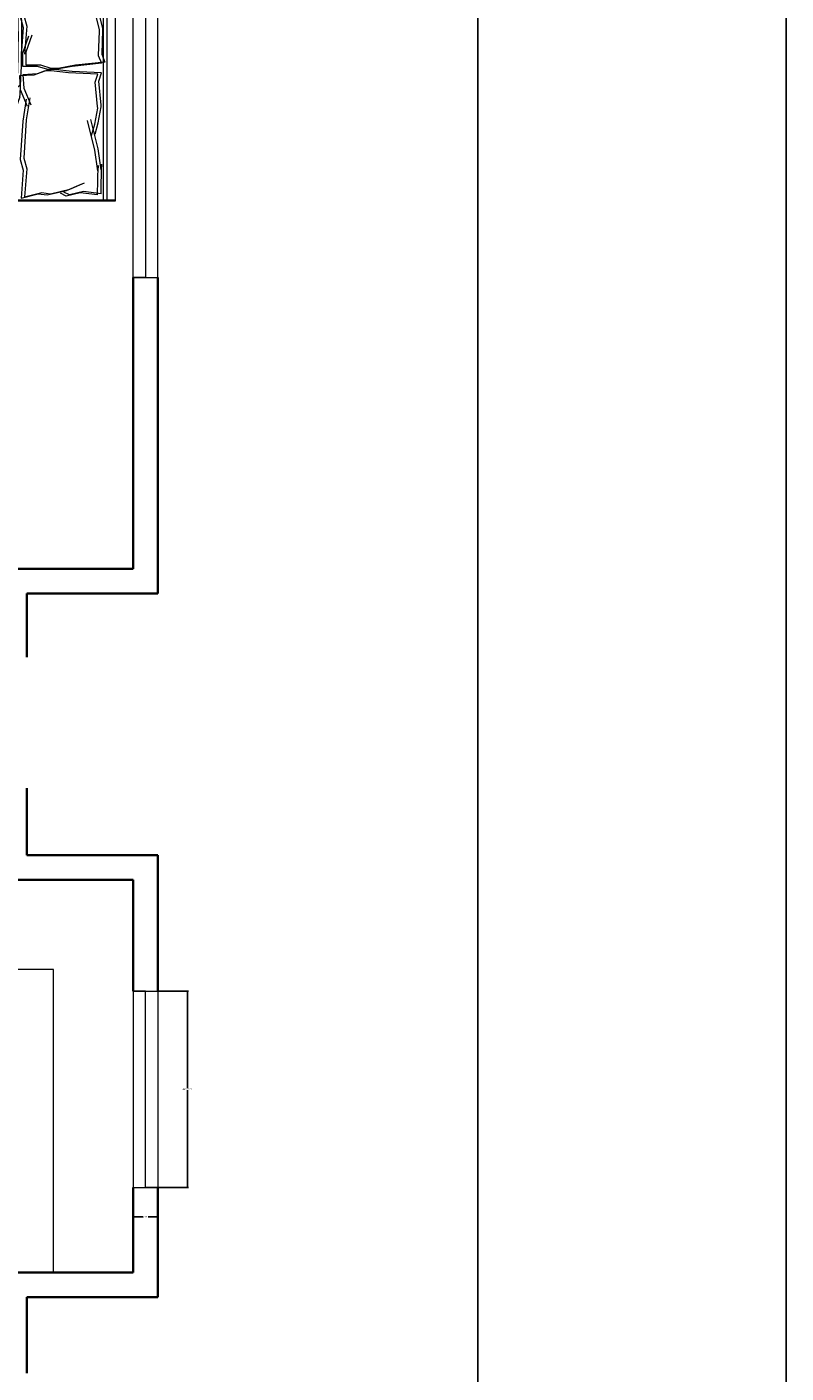
# Model space of a CAD drawing. Units: inches. Extents: x 2163 to 2982, y 1024 to 2288.
# Tile 8 of 22: x 2843 to 2982, y 1390 to 1637. Entities that reach past the tile are written whole.
import ezdxf

# ---------------------------------------------------------------- set-up
doc = ezdxf.new("R2010")
doc.units = ezdxf.units.IN
for name, color, linetype, lineweight in [('A-ANNO-DIMS', 2, 'Continuous', 18), ('A-ANNO-TTLB', 7, 'Continuous', 25), ('A-FLOR-FIXT', 9, 'Continuous', 18), ('A-FURN', 8, 'Continuous', 13), ('A-GLAZ', 161, 'Continuous', 18), ('A-WALL', 7, 'Continuous', 35)]:
    doc.layers.add(name, color=color, linetype=linetype, lineweight=lineweight)
doc.styles.get("Standard").update_dxf_attribs({"font": 'arial.ttf'})
doc.dimstyles.get("Standard").update_dxf_attribs({"dimtxt": 0.18, "dimasz": 0.18, "dimexe": 0.18, "dimexo": 0.0625, "dimgap": 0.09, "dimtad": 0, "dimtih": 1, "dimtoh": 1, "dimdec": 4, "dimzin": 0, "dimdsep": 46, "dimtxsty": 'Standard', "dimcen": 0.09, "dimadec": 0, "dimazin": 0, "dimtfac": 1, "dimtdec": 4, "dimtofl": 0, "dimtmove": 0, "dimatfit": 3, "dimfxl": 1, "dimtolj": 1, "dimtzin": 0, "dimarcsym": 0})

# ---------------------------------------------------------------- blocks, each defined once
blk = doc.blocks.new('BED-DOUBLE')
for p, q in [((27.75, 52.87), (24.5, 49.16)), ((27.75, 52.87), (24.5, 49.16)), ((28.38, 53.1), (25.13, 49.39)), ((28.38, 53.1), (25.13, 49.39)), ((29.49, 52.95), (27.75, 52.87, 3.87)), ((29.49, 52.95), (27.75, 52.87, 3.87)), ((28.36, 51.33), (27.75, 52.87)), ((28.36, 51.33), (27.75, 52.87)), ((30.13, 53.18), (28.38, 53.1, 3.87)), ((29, 51.56), (28.38, 53.1)), ((30.13, 53.18), (28.38, 53.1, 3.87)), ((29, 51.56), (28.38, 53.1)), ((0, 51.49), (0.64, 51.49)), ((0, 3.47), (0, 51.49)), ((0, 51.27), (26.61, 51.27)), ((0, 51.27), (26.61, 51.27)), ((0.64, 51.49), (27.25, 51.49)), ((0.64, 51.49), (27.25, 51.49)), ((1.53, 3.48), (1.53, 51.27)), ((1.53, 3.47), (1.53, 51.27)), ((2.17, 3.7), (2.17, 51.49)), ((2.17, 3.7), (2.17, 51.49)), ((2.56, 50.11), (2.46, 44.71)), ((2.56, 50.11), (2.46, 44.71)), ((2.56, 50.11), (5.77, 49.73)), ((2.56, 50.11), (5.77, 49.73)), ((3.2, 50.34), (3.1, 44.94)), ((3.2, 50.34), (3.1, 44.94)), ((3.2, 50.34), (6.41, 49.96)), ((3.2, 50.34), (6.41, 49.96)), ((5.77, 49.73), (8.34, 50.33)), ((5.77, 49.73), (8.34, 50.33)), ((8.9, 49.54), (6.22, 48.36)), ((8.9, 49.54), (6.22, 48.36)), ((6.41, 49.96), (8.98, 50.56)), ((6.41, 49.96), (8.98, 50.56)), ((11.83, 50.11), (8.26, 49.31)), ((11.83, 50.11), (8.26, 49.31)), ((8.34, 50.33), (9.38, 49.81)), ((8.34, 50.33), (9.38, 49.81)), ((12.47, 50.34), (8.9, 49.54)), ((12.47, 50.34), (8.9, 49.54)), ((8.98, 50.56), (10.02, 50.04)), ((8.98, 50.56), (10.02, 50.04)), ((13.43, 49.92), (11.83, 50.11)), ((13.43, 49.92), (11.83, 50.11)), ((14.07, 50.15), (12.47, 50.34)), ((14.07, 50.15), (12.47, 50.34)), ((16.57, 50.7), (13.43, 49.92)), ((16.57, 50.7), (13.43, 49.92)), ((17.21, 50.93), (14.07, 50.15)), ((17.21, 50.93), (14.07, 50.15)), ((16.17, 45.57), (16.57, 50.7)), ((16.17, 45.57), (16.57, 50.7)), ((16.81, 45.79), (17.21, 50.93)), ((16.81, 45.79), (17.21, 50.93)), ((25.13, 49.39), (22.97, 46.45)), ((25.13, 49.39), (22.97, 46.45)), ((28.06, 48.23), (28.36, 51.33)), ((28.06, 48.23), (28.36, 51.33)), ((28.69, 48.46), (29, 51.56)), ((28.69, 48.46), (29, 51.56)), ((8.26, 49.31), (5.58, 48.13)), ((8.26, 49.31), (5.58, 48.13)), ((24.5, 49.16), (22.33, 46.22)), ((24.5, 49.16), (22.33, 46.22)), ((28.36, 44.36), (28.06, 48.23)), ((28.36, 44.36), (28.06, 48.23)), ((29, 44.59), (28.69, 48.46)), ((29, 44.59), (28.69, 48.46)), ((2.46, 44.71), (2.54, 45.71)), ((2.46, 44.71), (2.54, 45.71)), ((2.54, 45.71), (3.07, 41.91)), ((2.54, 45.71), (3.07, 41.91)), ((3.1, 44.94), (3.18, 45.94)), ((3.1, 44.94), (3.18, 45.94)), ((3.18, 45.94), (3.71, 42.14)), ((3.18, 45.94), (3.71, 42.14)), ((16.73, 43.61), (16.17, 45.57)), ((16.73, 43.61), (16.17, 45.57)), ((17.37, 43.83), (16.81, 45.79)), ((17.37, 43.83), (16.81, 45.79)), ((22.33, 46.22), (20.32, 40.64)), ((22.33, 46.22), (20.32, 40.64)), ((22.97, 46.45), (20.96, 40.87)), ((22.97, 46.45), (20.96, 40.87)), ((29.47, 41.18), (29, 44.59)), ((29.47, 41.18), (29, 44.59)), ((3.71, 42.14), (5.06, 36.72)), ((3.71, 42.14), (5.06, 36.72)), ((16.29, 36.6), (16.73, 43.61)), ((16.29, 36.6), (16.73, 43.61)), ((16.93, 36.82), (17.37, 43.83)), ((16.93, 36.82), (17.37, 43.83)), ((28.83, 40.95), (28.36, 44.36)), ((28.83, 40.95), (28.36, 44.36)), ((3.07, 41.91), (4.42, 36.49)), ((3.07, 41.91), (4.42, 36.49)), ((20.32, 40.64), (17.38, 32.31)), ((20.32, 40.64), (17.38, 32.31)), ((20.96, 40.87), (18.02, 32.53)), ((20.96, 40.87), (18.02, 32.53)), ((29.76, 38.94), (28.83, 40.95)), ((29.76, 38.94), (28.83, 40.95)), ((30.4, 39.17), (29.47, 41.18)), ((30.4, 39.17), (29.47, 41.18)), ((79.24, 15.06), (79.24, 39.68)), ((79.24, 15.06), (79.24, 39.68)), ((79.88, 15.29), (79.88, 39.91)), ((79.88, 15.29), (79.88, 39.91)), ((3.08, 37.14), (2.54, 34.2)), ((3.08, 37.13), (2.54, 34.2)), ((3.67, 39.2), (3.08, 37.14)), ((3.67, 39.2), (3.08, 37.13)), ((3.72, 37.36), (3.18, 34.43)), ((3.72, 37.36), (3.18, 34.43)), ((4.31, 39.43), (3.72, 37.36)), ((4.31, 39.43), (3.72, 37.36)), ((30.38, 36.46), (29.76, 38.94)), ((30.38, 36.46), (29.76, 38.94)), ((31.02, 36.69), (30.4, 39.17)), ((31.02, 36.69), (30.4, 39.17)), ((15.63, 32.56), (16.29, 36.6)), ((15.63, 32.56), (16.29, 36.6)), ((16.27, 32.79), (16.93, 36.82)), ((16.27, 32.79), (16.93, 36.82)), ((18.02, 30.49), (24.52, 34.68)), ((18.02, 30.49), (24.52, 34.68)), ((23.88, 34.45), (28.36, 36.15)), ((23.88, 34.45), (28.36, 36.15)), ((24.52, 34.68), (29, 36.38)), ((24.52, 34.68), (29, 36.38)), ((28.36, 36.15), (30.38, 36.46)), ((28.36, 36.15), (30.38, 36.46)), ((29, 36.38), (31.02, 36.69)), ((29, 36.38), (31.02, 36.69)), ((2.54, 34.2), (2.56, 33.88)), ((2.54, 34.2), (2.56, 33.88)), ((2.56, 33.88), (2.98, 29.46)), ((2.56, 33.88), (2.98, 29.46)), ((3.18, 34.43), (3.2, 34.11)), ((3.18, 34.43), (3.2, 34.11)), ((3.2, 34.11), (3.62, 29.68)), ((3.2, 34.11), (3.62, 29.68)), ((16.74, 30.75), (15.45, 33.82)), ((16.74, 30.75), (15.45, 33.82)), ((17.38, 30.98), (16.09, 34.05)), ((17.38, 30.98), (16.09, 34.05)), ((17.38, 30.26), (23.88, 34.45)), ((17.38, 30.26), (23.88, 34.45)), ((3.62, 29.68), (3.13, 28.21)), ((3.62, 29.68), (3.13, 28.2)), ((16.89, 28.3), (16.74, 30.75)), ((16.89, 28.3), (16.74, 30.75)), ((17.53, 28.53), (17.38, 30.98)), ((17.53, 28.53), (17.38, 30.98)), ((2.98, 29.46), (2.49, 27.98)), ((2.98, 29.46), (2.49, 27.98)), ((2.49, 27.98), (7.87, 27.73)), ((2.49, 27.98), (7.87, 27.73)), ((3.13, 28.21), (8.51, 27.96)), ((3.13, 28.2), (8.51, 27.96)), ((7.86, 26.79), (11.04, 27.37)), ((7.86, 26.79), (11.04, 27.37)), ((7.87, 27.73), (11.08, 27.35)), ((7.87, 27.73), (11.08, 27.35)), ((8.51, 27.96), (11.72, 27.58)), ((8.51, 27.96), (11.72, 27.58)), ((11.04, 27.37), (12.34, 27.37)), ((11.04, 27.37), (12.34, 27.37)), ((11.08, 27.35), (12.38, 27.44)), ((11.08, 27.35), (12.38, 27.44)), ((11.72, 27.58), (13.02, 27.66)), ((11.72, 27.58), (13.02, 27.66)), ((12.34, 27.37), (14.22, 26.79)), ((12.34, 27.37), (14.22, 26.79)), ((12.38, 27.44), (14.22, 28.13)), ((12.38, 27.44), (14.22, 28.13)), ((13.02, 27.66), (14.86, 28.36)), ((13.02, 27.66), (14.86, 28.36)), ((14.22, 28.13), (16.89, 28.3)), ((14.22, 28.13), (16.89, 28.3)), ((14.86, 28.36), (17.53, 28.53)), ((14.86, 28.36), (17.53, 28.53)), ((1.87, 25.98), (7.22, 26.56)), ((1.87, 25.98), (7.22, 26.56)), ((2.45, 24.54), (1.87, 25.98)), ((2.45, 24.54), (1.87, 25.98)), ((2.51, 26.21), (7.86, 26.79)), ((2.51, 26.21), (7.86, 26.79)), ((3.09, 24.77), (2.51, 26.21)), ((3.09, 24.77), (2.51, 26.21)), ((2.94, 20.32), (3.09, 24.77)), ((2.94, 20.32), (3.09, 24.77)), ((7.22, 26.56), (10.4, 27.14)), ((7.22, 26.56), (10.4, 27.14)), ((10.4, 27.14), (11.7, 27.14)), ((10.4, 27.14), (11.7, 27.14)), ((11.7, 27.14), (13.58, 26.56)), ((11.7, 27.14), (13.58, 26.56)), ((13.58, 26.56), (16.26, 26.56)), ((13.58, 26.56), (16.26, 26.56)), ((14.22, 26.79), (16.9, 26.79)), ((14.22, 26.79), (16.9, 26.79)), ((16.26, 26.56), (16.26, 24.1)), ((16.26, 26.56), (16.26, 24.1)), ((16.81, 19.61), (17.21, 24.74)), ((16.81, 19.61), (17.21, 24.74)), ((16.9, 26.79), (16.9, 24.33)), ((16.9, 26.79), (16.9, 24.33)), ((2.3, 20.09), (2.45, 24.54)), ((2.3, 20.09), (2.45, 24.54)), ((16.26, 24.1), (15.17, 20.96)), ((16.26, 24.1), (15.17, 20.96)), ((16.9, 24.33), (15.81, 21.19)), ((16.9, 24.33), (15.81, 21.19)), ((16.17, 19.38), (16.57, 24.52)), ((16.17, 19.38), (16.57, 24.52)), ((2.3, 19.77), (2.3, 20.09)), ((2.3, 19.77), (2.3, 20.09)), ((3.03, 16.88), (2.3, 19.77)), ((3.03, 16.88), (2.3, 19.77)), ((2.94, 20), (2.94, 20.32)), ((2.94, 20), (2.94, 20.32)), ((3.67, 17.11), (2.94, 20)), ((3.67, 17.11), (2.94, 20)), ((3.32, 12.11), (4.33, 17.6)), ((3.32, 12.11), (4.33, 17.6)), ((3.96, 12.34), (4.97, 17.83)), ((3.96, 12.34), (4.97, 17.83)), ((16.73, 17.42), (16.17, 19.38)), ((16.73, 17.42), (16.17, 19.38)), ((16.29, 10.41), (16.73, 17.42)), ((16.29, 10.41), (16.73, 17.42)), ((17.37, 17.65), (16.81, 19.61)), ((17.37, 17.65), (16.81, 19.61)), ((16.93, 10.64), (17.37, 17.65)), ((16.93, 10.64), (17.37, 17.65)), ((3.75, 14.85), (3.03, 16.88)), ((3.75, 14.85), (3.03, 16.88)), ((4.39, 15.08), (3.67, 17.11)), ((4.39, 15.08), (3.67, 17.11)), ((3.03, 8.28), (3.32, 12.11)), ((3.03, 8.28), (3.32, 12.11)), ((3.67, 8.51), (3.96, 12.34)), ((3.67, 8.51), (3.96, 12.34)), ((15.63, 6.38), (16.29, 10.41)), ((15.63, 6.38), (16.29, 10.41)), ((16.27, 6.61), (16.93, 10.64)), ((16.27, 6.61), (16.93, 10.64)), ((16.29, 10.41), (16.62, 9.28)), ((16.29, 10.41), (16.62, 9.28)), ((16.93, 10.64), (17.26, 9.51)), ((16.93, 10.64), (17.26, 9.51)), ((3.01, 8.18), (3.03, 8.28)), ((3.01, 8.18), (3.03, 8.28)), ((3.34, 3.9), (3.01, 8.18)), ((3.34, 3.9), (3.01, 8.18)), ((3.65, 8.41), (3.67, 8.51)), ((3.65, 8.41), (3.67, 8.51)), ((3.98, 4.13), (3.65, 8.41)), ((3.98, 4.13), (3.65, 8.41)), ((16.62, 9.28), (17.34, 4.18)), ((16.62, 9.28), (17.34, 4.18)), ((17.26, 9.51), (17.98, 4.41)), ((17.26, 9.51), (17.98, 4.41)), ((8.95, 5.05), (6.21, 6.06)), ((8.95, 5.05), (6.21, 6.06)), ((9.59, 5.28), (6.85, 6.29)), ((9.59, 5.28), (6.85, 6.29)), ((12.57, 4.47), (8.95, 5.05)), ((12.57, 4.47), (8.95, 5.05)), ((13.21, 4.7), (9.59, 5.28)), ((13.21, 4.7), (9.59, 5.28)), ((14.8, 4.99), (13.21, 4.7)), ((14.8, 4.99), (13.21, 4.7)), ((17.98, 4.41), (14.8, 4.99)), ((17.98, 4.41), (14.8, 4.99)), ((18.11, 3.48), (0, 3.48)), ((18.11, 3.47), (0, 3.47)), ((18.75, 3.7), (0.64, 3.7)), ((18.75, 3.7), (0.64, 3.7)), ((3.32, 3.89), (6.5, 4.47)), ((3.32, 3.89), (6.5, 4.47)), ((3.96, 4.12), (7.14, 4.7)), ((3.96, 4.12), (7.14, 4.7)), ((6.5, 4.47), (9.1, 4.04)), ((6.5, 4.47), (9.1, 4.04)), ((7.14, 4.7), (9.74, 4.27)), ((7.14, 4.7), (9.74, 4.27)), ((9.1, 4.04), (10.11, 4.62)), ((9.1, 4.04), (10.11, 4.62)), ((9.74, 4.27), (10.75, 4.85)), ((9.74, 4.27), (10.75, 4.85)), ((14.16, 4.76), (12.57, 4.47)), ((14.16, 4.76), (12.57, 4.47)), ((17.34, 4.18), (14.16, 4.76)), ((17.34, 4.18), (14.16, 4.76))]:
    blk.add_line(p, q)
for centre, radius, start, end in [((68.67, 76.16), 23.07, 267.4714, 296.4681), ((68.67, 76.16), 23.07, 267.4714, 296.4681), ((69.31, 76.39), 23.07, 267.4714, 296.4681), ((69.31, 76.39), 23.07, 267.4714, 296.4681), ((78.87, 54.41), 1.1, 332.6588, 86.02), ((78.87, 54.41), 1.1, 332.6588, 86.02), ((79.51, 54.64), 1.1, 332.6588, 86.02), ((79.51, 54.64), 1.1, 332.6588, 86.02), ((-6.66, 51.33), 36.18, 349.8763, 2.5657), ((-6.66, 51.33), 36.18, 349.8763, 2.5657), ((36.31, 182.27), 129.5, 266.9791, 273.8365), ((36.31, 182.27), 129.5, 266.9791, 273.8365), ((-6.02, 51.56), 36.18, 349.8763, 2.5657), ((-6.02, 51.56), 36.18, 349.8763, 2.5657), ((36.95, 182.49), 129.5, 266.9791, 273.8365), ((36.95, 182.49), 129.5, 266.9791, 273.8365), ((67.82, -4508.74), 4561.86, 90.00217, 90.28689), ((67.82, -4508.74), 4561.86, 90.00217, 90.28689), ((68.46, -4508.52), 4561.86, 90.00217, 90.28689), ((68.46, -4508.52), 4561.86, 90.00217, 90.28689), ((212.28, 41.15), 133.04, 174.4998, 180.6351), ((212.28, 41.15), 133.04, 174.4998, 180.6351), ((212.92, 41.38), 133.04, 174.4998, 180.6351), ((212.92, 41.38), 133.04, 174.4998, 180.6351), ((35.07, 43.74), 6.22, 168.6608, 203.7384), ((35.07, 43.74), 6.22, 168.6608, 203.7384), ((35.71, 43.97), 6.22, 168.6608, 203.7384), ((35.71, 43.97), 6.22, 168.6608, 203.7384), ((1.48, 31.15), 29.65, 10.6617, 19.8806), ((1.48, 31.15), 29.65, 10.6617, 19.8806), ((2.12, 31.38), 29.65, 10.6617, 19.8806), ((2.12, 31.38), 29.65, 10.6617, 19.8806), ((156.32, 17.76), 129.02, 171.7845, 186.9006), ((156.32, 17.76), 129.02, 171.7845, 186.9006), ((156.96, 17.98), 129.02, 171.7845, 186.9006), ((156.96, 17.98), 129.02, 171.7845, 186.9006), ((30.44, 36.64), 0.185, 250.2464, 1.1377), ((30.44, 36.64), 0.185, 250.2464, 1.1377), ((31.08, 36.86), 0.185, 250.2464, 1.1377), ((31.08, 36.86), 0.185, 250.2464, 1.1377), ((182.05, 21.36), 164.97, 176.0865, 186.7821), ((182.05, 21.36), 164.97, 176.0865, 186.7821), ((182.69, 21.59), 164.97, 176.0865, 186.7821), ((182.69, 21.59), 164.97, 176.0865, 186.7821), ((-23.71, -17.22), 106.46, 13.3832, 17.7053), ((-23.71, -17.22), 106.46, 13.3832, 17.7053), ((-23.07, -16.99), 106.46, 13.3832, 17.7053), ((-23.07, -16.99), 106.46, 13.3832, 17.7053), ((200.84, 21.43), 121.76, 182.9958, 189.4091), ((200.84, 21.43), 121.76, 182.9958, 189.4091), ((201.48, 21.66), 121.76, 182.9958, 189.4091), ((201.48, 21.65), 121.76, 182.9958, 189.4091), ((20.74, 85.39), 83.31, 268.7218, 275.604), ((20.74, 85.39), 83.31, 268.7218, 275.604), ((31.17, -167.31), 170.11, 88.4762, 91.0082), ((31.17, -167.31), 170.11, 88.4762, 91.0082), ((31.81, -167.08), 170.11, 88.4762, 91.0082), ((31.81, -167.08), 170.11, 88.4762, 91.0082), ((50.61, 484.82), 482.31, 268.2277, 271.7185), ((50.61, 484.82), 482.31, 268.2277, 271.7185), ((51.25, 485.05), 482.31, 268.2277, 271.7185), ((51.25, 485.05), 482.31, 268.2277, 271.7185), ((64.51, -26.9), 29.63, 76.0648, 88.9113), ((64.51, -26.9), 29.63, 76.0648, 88.9113), ((65.15, -26.67), 29.63, 76.0648, 88.9113), ((65.15, -26.67), 29.63, 76.0648, 88.9113), ((20.1, 85.16), 83.31, 268.7218, 275.604), ((20.1, 85.16), 83.31, 268.7218, 275.604), ((70.28, -21.66), 23.56, 67.9751, 86.652), ((70.28, -21.66), 23.56, 67.9751, 86.652), ((70.91, -21.43), 23.56, 67.9751, 86.652), ((70.91, -21.43), 23.56, 67.9751, 86.652), ((79.72, 1.09), 1.09, 236.1736, 23.4781), ((79.72, 1.09), 1.09, 236.1736, 23.4781), ((80.36, 1.32), 1.09, 236.1736, 23.4781), ((80.36, 1.32), 1.09, 236.1736, 23.4781)]:
    blk.add_arc(centre, radius, start, end)
blk = doc.blocks.new('WIN-60')
for p, q in [((2.25, 60), (0, 60)), ((0, 60), (4.5, 60)), ((0, 60), (0, 0)), ((2.25, 0), (2.25, 60)), ((4.5, 60), (4.5, 0)), ((0, 0), (4.5, 0)), ((4.5, 0), (2.25, 0))]:
    blk.add_line(p, q)
blk = doc.blocks.new('WIN-36')
for p, q in [((2.25, 36), (0, 36)), ((0, 36), (4.5, 36)), ((0, 36), (0, 0)), ((2.25, 0), (2.25, 36)), ((4.5, 36), (4.5, 0)), ((0, 0), (4.5, 0)), ((4.5, 0), (2.25, 0))]:
    blk.add_line(p, q)
blk = doc.blocks.new('*D15')
at = {"layer": 'A-ANNO-DIMS', "color": 0, "lineweight": -2, "transparency": 16777216}
for p, q in [((2867.4, 1460.37), (2872.92, 1460.37)), ((2872.74, 1460.19), (2872.74, 1442.56)), ((2872.74, 1424.55), (2872.74, 1442.19)), ((2867.4, 1424.37), (2872.92, 1424.37))]:
    blk.add_line(p, q, dxfattribs=at)
at = {"layer": 'A-ANNO-DIMS', "color": 0, "transparency": 16777216}
for points in [[(2872.71, 1460.19), (2872.77, 1460.19), (2872.74, 1460.37)], [(2872.71, 1424.55), (2872.77, 1424.55), (2872.74, 1424.37)]]:
    blk.add_solid(points, dxfattribs=at)
at = {"layer": 'Defpoints', "color": 0, "transparency": 16777216}
for p in [(2867.34, 1460.37), (2872.74, 1460.37), (2867.34, 1424.37)]:
    blk.add_point(p, dxfattribs=at)
at = {"layer": 'A-ANNO-DIMS', "color": 0, "transparency": 16777216, "insert": (2872.74, 1442.37), "char_height": 0.18, "attachment_point": 5}
blk.add_mtext('\\A1;WINDOW 36 TYP.', dxfattribs=at)
blk = doc.blocks.new('*D16')
at = {"layer": 'A-ANNO-DIMS', "color": 0, "lineweight": -2, "transparency": 16777216}
for p, q in [((2862.84, 1424.31), (2862.84, 1418.79)), ((2867.34, 1424.31), (2867.34, 1418.79)), ((2863.02, 1418.97), (2864.63, 1418.97)), ((2867.16, 1418.97), (2865.55, 1418.97))]:
    blk.add_line(p, q, dxfattribs=at)
at = {"layer": 'A-ANNO-DIMS', "color": 0, "transparency": 16777216}
for points in [[(2863.02, 1419), (2863.02, 1418.94), (2862.84, 1418.97)], [(2867.16, 1419), (2867.16, 1418.94), (2867.34, 1418.97)]]:
    blk.add_solid(points, dxfattribs=at)
at = {"layer": 'Defpoints', "color": 0, "transparency": 16777216}
for p in [(2862.84, 1424.37), (2867.34, 1424.37), (2867.34, 1418.97)]:
    blk.add_point(p, dxfattribs=at)
at = {"layer": 'A-ANNO-DIMS', "color": 0, "transparency": 16777216, "insert": (2865.09, 1418.97), "char_height": 0.18, "attachment_point": 5}
blk.add_mtext('\\A1;5 TYP.', dxfattribs=at)
blk = doc.blocks.new('*D32')
at = {"layer": 'A-ANNO-DIMS', "color": 0, "lineweight": -2, "transparency": 16777216}
for p, q in [((2867.4, 2229.27), (2926.17, 2229.27)), ((2925.99, 2229.09), (2925.99, 1686.35)), ((2925.99, 1143.25), (2925.99, 1685.99)), ((2867.4, 1143.07), (2926.17, 1143.07))]:
    blk.add_line(p, q, dxfattribs=at)
at = {"layer": 'A-ANNO-DIMS', "color": 0, "transparency": 16777216}
for points in [[(2925.96, 2229.09), (2926.02, 2229.09), (2925.99, 2229.27)], [(2925.96, 1143.25), (2926.02, 1143.25), (2925.99, 1143.07)]]:
    blk.add_solid(points, dxfattribs=at)
at = {"layer": 'Defpoints', "color": 0, "transparency": 16777216}
for p in [(2867.34, 2229.27), (2925.99, 2229.27), (2867.34, 1143.07)]:
    blk.add_point(p, dxfattribs=at)
at = {"layer": 'A-ANNO-DIMS', "color": 0, "transparency": 16777216, "insert": (2925.99, 1686.17), "char_height": 0.18, "attachment_point": 5}
blk.add_mtext('\\A1;1086.2', dxfattribs=at)

msp = doc.modelspace()

# ---------------------------------------------------------------- linework, layer by layer
at = {"layer": 'A-ANNO-TTLB'}
msp.add_lwpolyline([(2162.6841, 2274.6054), (2982.469, 2274.6054), (2982.469, 1045.9691), (2162.6841, 1045.9691)], close=True, dxfattribs=at)
at = {"layer": 'A-FLOR-FIXT'}
for p, q in [((2848.1781, 1464.335), (2718.8389, 1464.335)), ((2848.1781, 1408.7688), (2848.1781, 1464.335))]:
    msp.add_line(p, q, dxfattribs=at)
at = {"layer": 'A-WALL'}
for p, q in [((2862.8389, 1591.1733), (2862.8389, 1537.7688)), ((2867.3389, 1591.1733), (2867.3389, 1533.2688)), ((2718.8389, 1537.7688), (2862.8389, 1537.7688)), ((2867.3389, 1533.2688), (2843.3389, 1533.2688)), ((2843.3389, 1533.2688), (2862.8389, 1533.2688)), ((2843.3389, 1521.5742), (2843.3389, 1533.2688)), ((2843.3389, 1485.2688), (2843.3389, 1497.5742)), ((2843.3389, 1485.2688), (2867.3389, 1485.2688)), ((2867.3389, 1485.2688), (2867.3389, 1460.3737)), ((2718.8389, 1480.7688), (2862.8389, 1480.7688)), ((2862.8389, 1480.7688), (2862.8389, 1460.3737)), ((2862.8389, 1424.3737), (2862.8389, 1408.7688)), ((2867.3389, 1424.3737), (2867.3389, 1404.2688)), ((2744.1034, 1408.7688), (2862.8389, 1408.7688)), ((2843.3389, 1404.2688), (2843.3389, 1390.3249)), ((2843.3389, 1404.2688), (2867.3389, 1404.2688))]:
    msp.add_line(p, q, dxfattribs=at)

# ---------------------------------------------------------------- block references
at = {"layer": 'A-FURN', "rotation": 180}
msp.add_blockref('BED-DOUBLE', (2859.4875, 1656.6782), dxfattribs=at)
at = {"layer": 'A-GLAZ', "extrusion": (0, 0, -1), "zscale": -1, "rotation": 180}
msp.add_blockref('WIN-60', (-2862.839, 1651.1734), dxfattribs=at)
at = {"layer": 'A-GLAZ'}
msp.add_blockref('WIN-36', (2862.839, 1424.3733), dxfattribs=at)

# ---------------------------------------------------------------- dimensions: what is measured, and where the dimension line sits
at = {"layer": 'A-ANNO-DIMS'}
dim = msp.add_linear_dim(base=(2925.9889, 2229.2688), p1=(2867.3389, 1143.0732), p2=(2867.3389, 2229.2688), angle=90, dimstyle='Standard', override={"dimdec": 1, "dimlfac": 1, "dimrnd": 0, "dimzin": 0, "dimdsep": 46, "dimlunit": 2}, dxfattribs=at)
dim.commit()
dim.dimension.update_dxf_attribs({"geometry": '*D32', "text_midpoint": (2925.9889, 1686.171)})
dim = msp.add_linear_dim(base=(2872.7389, 1460.3737), p1=(2867.3389, 1424.3737), p2=(2867.3389, 1460.3737), angle=90, text='WINDOW <> TYP.', dimstyle='Standard', override={"dimdec": 0, "dimlfac": 1, "dimrnd": 0, "dimzin": 0, "dimdsep": 46, "dimlunit": 2}, dxfattribs=at)
dim.commit()
dim.dimension.update_dxf_attribs({"geometry": '*D15', "text_midpoint": (2872.7389, 1442.3737)})
dim = msp.add_linear_dim(base=(2867.3389150341, 1418.9736749216), p1=(2862.8389150341, 1424.3736749216), p2=(2867.3389150341, 1424.3736749216), text='<> TYP.', dimstyle='Standard', override={"dimdec": 0, "dimlfac": 1, "dimrnd": 0, "dimzin": 0, "dimdsep": 46, "dimlunit": 2}, dxfattribs=at)
dim.commit()
dim.dimension.update_dxf_attribs({"geometry": '*D16', "text_midpoint": (2865.0889150341, 1418.9736749216)})

doc.saveas('drawing.dxf')
